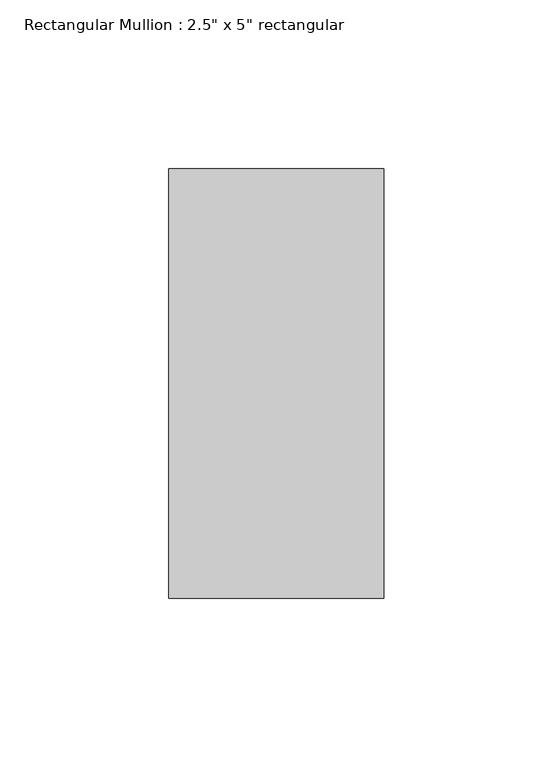
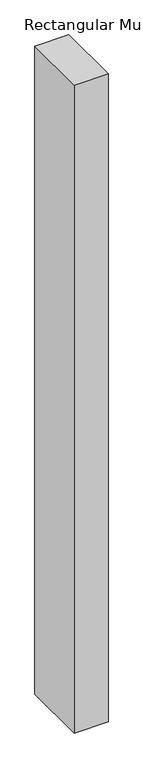
"""IFC4 building model written with IfcOpenShell, lengths in millimetres: member geometry."""

from ifc_helpers import new_model, si_unit, frame, origin, place, context, project, spatial, polyline, outline, extrude, source, transform, mapped, element, save


def member_7824d57a(model_context):
    return source(origin(), model_context, "Body", "SweptSolid", [
        extrude(outline(polyline([(31.75, 63.5), (31.75, -63.5), (-31.75, -63.5), (-31.75, 63.5), (31.75, 63.5)])), frame((0.0, 0.0, -1281.4606784), z_axis=(0.0, 0.0, 1.0), x_axis=(1.0, 0.0, 0.0)), (0.0, 0.0, 1.0), 1281.4606784),
    ])


if __name__ == "__main__":
    model = new_model("IFC4")
    model_context = context("Model", 3, world=origin())
    ifc_project = project(units=[si_unit("LENGTHUNIT", "METRE", prefix="MILLI")], contexts=[model_context])
    site = spatial("IfcSite", under=ifc_project)
    building = spatial("IfcBuilding", under=site)
    placement = place(None, origin())
    member_shape = member_7824d57a(model_context)
    element("IfcMember", 1, ObjectType="Rectangular Mullion : 2.5\" x 5\" rectangular", at=placement, inside=building, context=model_context, shape_type="MappedRepresentation", body=[
        mapped(member_shape, transform((0.0, 0.0, 0.0), x_axis=(1.0, 0.0, 0.0), y_axis=(0.0, 1.0, 0.0), z_axis=(0.0, 0.0, 1.0))),
    ])
    save(model, "model.ifc")

# Revit data of these elements
# Type "Rectangular Mullion : 2.5\" x 5\" rectangular"
#   built-in parameter 1007304 = 0.416667 (stored number, unit not read)
#   built-in parameter 1007301 = 0.104167 (stored number, unit not read)
#   built-in parameter 1007300 = 0.104167 (stored number, unit not read)
# Element 1 (IfcMember, "Rectangular Mullion : 2.5\" x 5\" rectangular")
#   Materials on its faces: "Aluminum"
# Materials
#   "Aluminum": class "Metal", colour RGB 247 247 247, transparency 0, Description = "Aluminum 6061", Cost = 0
